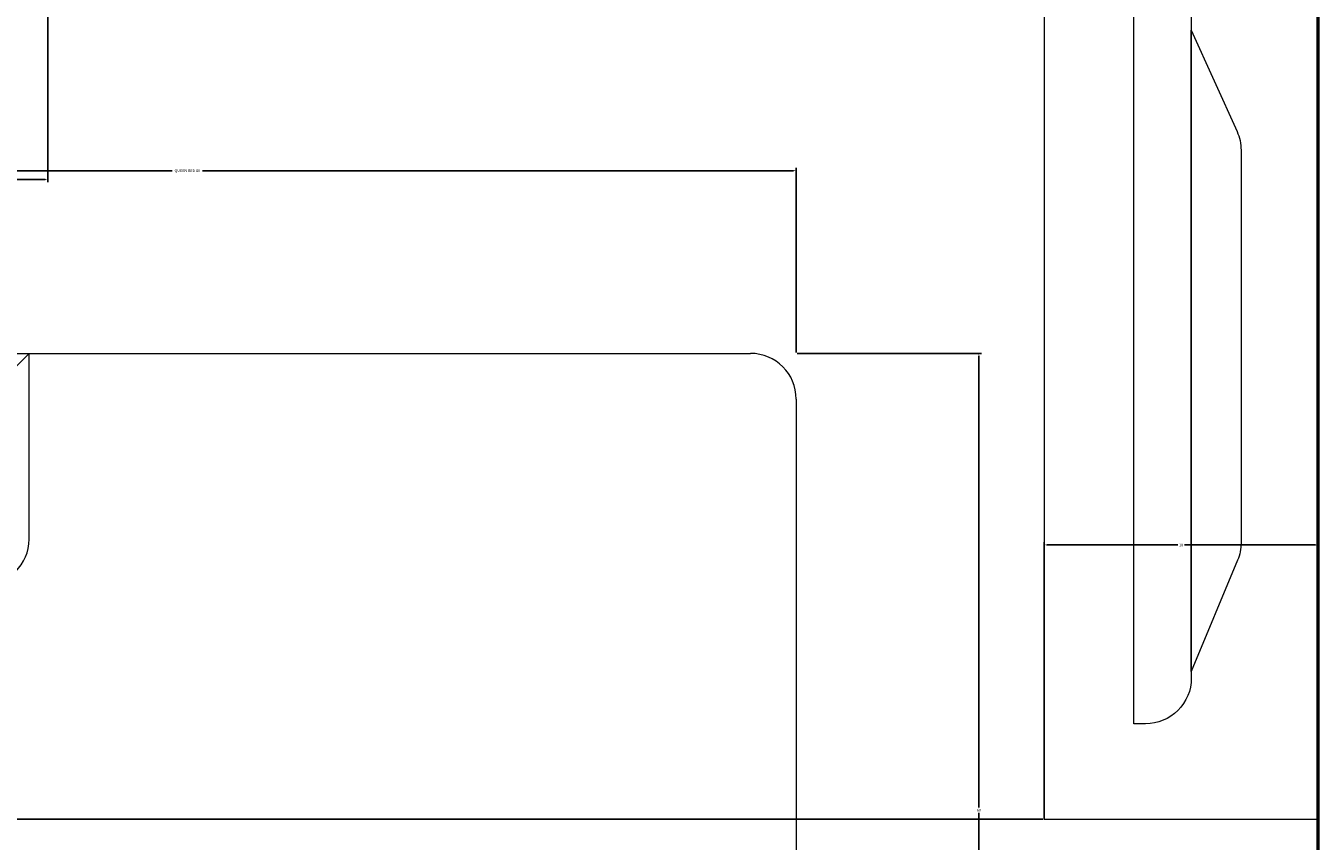
# Model space of a CAD drawing. Units: inches. Extents: x 2621 to 2849, y 2066 to 2463.
# Tile 17 of 28: x 2679 to 2764, y 2374 to 2427. Entities that reach past the tile are written whole.
import ezdxf

# ---------------------------------------------------------------- set-up
doc = ezdxf.new("R2010")
doc.units = ezdxf.units.IN
for name, color, linetype, lineweight in [('A-ANNO-DIMS', 2, 'Continuous', 18), ('A-EQPM', 8, 'Continuous', 18), ('A-FURN', 8, 'Continuous', 18), ('A-WALL', 7, 'Continuous', 50)]:
    doc.layers.add(name, color=color, linetype=linetype, lineweight=lineweight)
doc.styles.get("Standard").update_dxf_attribs({"font": 'arial.ttf'})
doc.dimstyles.get("Standard").update_dxf_attribs({"dimtxt": 0.18, "dimasz": 0.18, "dimexe": 0.18, "dimexo": 0.0625, "dimgap": 0.09, "dimtad": 0, "dimtih": 1, "dimtoh": 1, "dimdec": 4, "dimzin": 0, "dimdsep": 46, "dimtxsty": 'Standard', "dimcen": 0.09, "dimadec": 0, "dimazin": 0, "dimtfac": 1, "dimtdec": 4, "dimtofl": 0, "dimtmove": 0, "dimatfit": 3, "dimfxl": 1, "dimtolj": 1, "dimtzin": 0, "dimarcsym": 0})

# ---------------------------------------------------------------- blocks, each defined once
blk = doc.blocks.new('Bed - Queen')
for p, q in [((59.99999, -3), (59.99999, -77.00003)), ((59.99999, -29.6), (44.8, -14.4)), ((47.8, -29.6), (59.99999, -29.6)), ((56.99999, -80.00003), (3, -80.00003))]:
    blk.add_line(p, q)
for centre, start, end in [((47.8, -26.6), 180, 270), ((56.99999, -77.00003), 270, 0)]:
    blk.add_arc(centre, 3, start, end)
blk = doc.blocks.new('*D15')
at = {"layer": 'A-ANNO-DIMS', "color": 0, "lineweight": -2, "transparency": 16777216}
for p, q in [((2649.581, 2406.016), (2649.581, 2418.134)), ((2729.581, 2406.016), (2729.581, 2418.134)), ((2649.761, 2417.954), (2688.587, 2417.954)), ((2729.401, 2417.954), (2690.575, 2417.954))]:
    blk.add_line(p, q, dxfattribs=at)
at = {"layer": 'A-ANNO-DIMS', "color": 0, "transparency": 16777216}
for points in [[(2649.761, 2417.984), (2649.761, 2417.924), (2649.581, 2417.954)], [(2729.401, 2417.984), (2729.401, 2417.924), (2729.581, 2417.954)]]:
    blk.add_solid(points, dxfattribs=at)
at = {"layer": 'Defpoints', "color": 0, "transparency": 16777216}
for p in [(2649.581, 2417.954), (2649.581, 2405.954), (2729.581, 2405.954)]:
    blk.add_point(p, dxfattribs=at)
at = {"layer": 'A-ANNO-DIMS', "color": 0, "transparency": 16777216, "insert": (2689.581, 2417.954), "char_height": 0.18, "attachment_point": 5}
blk.add_mtext('\\A1;QUEEN BED 80', dxfattribs=at)
blk = doc.blocks.new('*D16')
at = {"layer": 'A-ANNO-DIMS', "color": 0, "lineweight": -2, "transparency": 16777216}
for p, q in [((2729.644, 2405.954), (2741.761, 2405.954)), ((2741.581, 2405.774), (2741.581, 2376.136)), ((2741.581, 2346.134), (2741.581, 2375.772)), ((2729.644, 2345.954), (2741.761, 2345.954))]:
    blk.add_line(p, q, dxfattribs=at)
at = {"layer": 'A-ANNO-DIMS', "color": 0, "transparency": 16777216}
for points in [[(2741.551, 2405.774), (2741.611, 2405.774), (2741.581, 2405.954)], [(2741.551, 2346.134), (2741.611, 2346.134), (2741.581, 2345.954)]]:
    blk.add_solid(points, dxfattribs=at)
at = {"layer": 'Defpoints', "color": 0, "transparency": 16777216}
for p in [(2729.581, 2405.954), (2741.581, 2405.954), (2729.581, 2345.954)]:
    blk.add_point(p, dxfattribs=at)
at = {"layer": 'A-ANNO-DIMS', "color": 0, "transparency": 16777216, "insert": (2741.581, 2375.954), "char_height": 0.18, "attachment_point": 5}
blk.add_mtext('\\A1;60', dxfattribs=at)
blk = doc.blocks.new('*D37')
at = {"layer": 'A-ANNO-DIMS', "color": 0, "lineweight": -2, "transparency": 16777216}
for p, q in [((2647.87, 2435.312), (2647.87, 2417.191)), ((2680.422, 2435.312), (2680.422, 2417.191)), ((2648.05, 2417.371), (2663.752, 2417.371)), ((2680.242, 2417.371), (2664.54, 2417.371))]:
    blk.add_line(p, q, dxfattribs=at)
at = {"layer": 'A-ANNO-DIMS', "color": 0, "transparency": 16777216}
for points in [[(2648.05, 2417.401), (2648.05, 2417.341), (2647.87, 2417.371)], [(2680.242, 2417.401), (2680.242, 2417.341), (2680.422, 2417.371)]]:
    blk.add_solid(points, dxfattribs=at)
at = {"layer": 'Defpoints', "color": 0, "transparency": 16777216}
for p in [(2647.87, 2435.375), (2680.422, 2435.375), (2647.87, 2417.371)]:
    blk.add_point(p, dxfattribs=at)
at = {"layer": 'A-ANNO-DIMS', "color": 0, "transparency": 16777216, "insert": (2664.146, 2417.371), "char_height": 0.18, "attachment_point": 5}
blk.add_mtext('\\A1;32.55', dxfattribs=at)
blk = doc.blocks.new('*D67')
at = {"layer": 'A-ANNO-DIMS', "color": 0, "lineweight": -2, "transparency": 16777216}
for p, q in [((2745.87, 2375.437), (2745.87, 2393.558)), ((2746.05, 2393.378), (2754.659, 2393.378)), ((2763.69, 2393.378), (2755.081, 2393.378)), ((2763.87, 2375.437), (2763.87, 2393.558))]:
    blk.add_line(p, q, dxfattribs=at)
at = {"layer": 'A-ANNO-DIMS', "color": 0, "transparency": 16777216}
for points in [[(2746.05, 2393.408), (2746.05, 2393.348), (2745.87, 2393.378)], [(2763.69, 2393.408), (2763.69, 2393.348), (2763.87, 2393.378)]]:
    blk.add_solid(points, dxfattribs=at)
at = {"layer": 'Defpoints', "color": 0, "transparency": 16777216}
for p in [(2763.87, 2393.378), (2745.87, 2375.375), (2763.87, 2375.375)]:
    blk.add_point(p, dxfattribs=at)
at = {"layer": 'A-ANNO-DIMS', "color": 0, "transparency": 16777216, "insert": (2754.87, 2393.378), "char_height": 0.18, "attachment_point": 5}
blk.add_mtext('\\A1;18', dxfattribs=at)
blk = doc.blocks.new('*D68')
at = {"layer": 'A-ANNO-DIMS', "color": 0, "lineweight": -2, "transparency": 16777216}
for p, q in [((2745.808, 2435.375), (2620.687, 2435.375)), ((2620.867, 2435.195), (2620.867, 2405.556)), ((2620.867, 2375.555), (2620.867, 2405.193)), ((2745.808, 2375.375), (2620.687, 2375.375))]:
    blk.add_line(p, q, dxfattribs=at)
at = {"layer": 'A-ANNO-DIMS', "color": 0, "transparency": 16777216}
for points in [[(2620.837, 2435.195), (2620.897, 2435.195), (2620.867, 2435.375)], [(2620.837, 2375.555), (2620.897, 2375.555), (2620.867, 2375.375)]]:
    blk.add_solid(points, dxfattribs=at)
at = {"layer": 'Defpoints', "color": 0, "transparency": 16777216}
for p in [(2620.867, 2435.375), (2745.87, 2435.375), (2745.87, 2375.375)]:
    blk.add_point(p, dxfattribs=at)
at = {"layer": 'A-ANNO-DIMS', "color": 0, "transparency": 16777216, "insert": (2620.867, 2405.375), "char_height": 0.18, "attachment_point": 5}
blk.add_mtext('\\A1;60', dxfattribs=at)

msp = doc.modelspace()

# ---------------------------------------------------------------- linework, layer by layer
at = {"layer": 'A-EQPM'}
msp.add_lwpolyline([(2751.7541, 2431.1293), (2752.5373, 2431.1293, -0.4142136), (2755.5373, 2428.1293), (2755.5373, 2384.6294, -0.4142136), (2752.5373, 2381.6294), (2751.7541, 2381.6294)], format="xyb", close=True, dxfattribs=at)
msp.add_lwpolyline([(2755.5373, 2427.1762), (2758.5388, 2420.5301, -0.1064481), (2758.8047, 2419.2954), (2758.8047, 2393.5184, -0.0988987), (2758.5744, 2392.3658), (2755.5373, 2385.0669)], format="xyb", dxfattribs=at)
msp.add_lwpolyline([(2755.5373, 2385.0669), (2755.5373, 2427.1762)], dxfattribs=at)
at = {"layer": 'A-FURN'}
msp.add_lwpolyline([(2763.8701, 2435.3746), (2745.8701, 2435.3746), (2745.8701, 2375.3746), (2763.8701, 2375.3746)], close=True, dxfattribs=at)
at = {"layer": 'A-WALL'}
msp.add_line((2763.8701, 2355.3746), (2763.8701, 2435.3746), dxfattribs=at)

# ---------------------------------------------------------------- block references
at = {"layer": 'A-FURN', "rotation": 90}
msp.add_blockref('Bed - Queen', (2649.5811, 2345.9537), dxfattribs=at)

# ---------------------------------------------------------------- dimensions: what is measured, and where the dimension line sits
at = {"layer": 'A-ANNO-DIMS'}
for base, p1, p2, angle, override, picture, middle in [((2620.8666, 2435.3746), (2745.8701, 2375.3746), (2745.8701, 2435.3746), 90, {"dimdec": 0, "dimlfac": 1, "dimrnd": 0, "dimzin": 0, "dimdsep": 46, "dimlunit": 2}, '*D68', (2620.8666, 2405.3746)), ((2647.8701, 2417.3711), (2680.4219, 2435.3746), (2647.8701, 2435.3746), 180, {"dimdec": 2, "dimlfac": 1, "dimrnd": 0, "dimzin": 0, "dimdsep": 46, "dimlunit": 2}, '*D37', (2664.146, 2417.3711)), ((2741.5811, 2405.9537), (2729.5811, 2345.9537), (2729.5811, 2405.9537), 90, {"dimdec": 0, "dimlfac": 1, "dimrnd": 0, "dimzin": 0, "dimdsep": 46, "dimlunit": 2}, '*D16', (2741.5811, 2375.9537))]:
    dim = msp.add_linear_dim(base=base, p1=p1, p2=p2, angle=angle, dimstyle='Standard', override=override, dxfattribs=at)
    dim.commit()
    dim.dimension.update_dxf_attribs({"geometry": picture, "text_midpoint": middle})
dim = msp.add_linear_dim(base=(2649.5811, 2417.9537), p1=(2729.5811, 2405.9537), p2=(2649.5811, 2405.9537), angle=180, text='QUEEN BED <>', dimstyle='Standard', override={"dimdec": 0, "dimlfac": 1, "dimrnd": 0, "dimzin": 0, "dimdsep": 46, "dimlunit": 2}, dxfattribs=at)
dim.commit()
dim.dimension.update_dxf_attribs({"geometry": '*D15', "text_midpoint": (2689.5811, 2417.9537)})
dim = msp.add_linear_dim(base=(2763.8701, 2393.3781), p1=(2745.8701, 2375.3746), p2=(2763.8701, 2375.3746), dimstyle='Standard', override={"dimdec": 0, "dimlfac": 1, "dimrnd": 0, "dimzin": 0, "dimdsep": 46, "dimlunit": 2}, dxfattribs=at)
dim.commit()
dim.dimension.update_dxf_attribs({"geometry": '*D67', "text_midpoint": (2754.8701, 2393.3781)})

doc.saveas('drawing.dxf')
